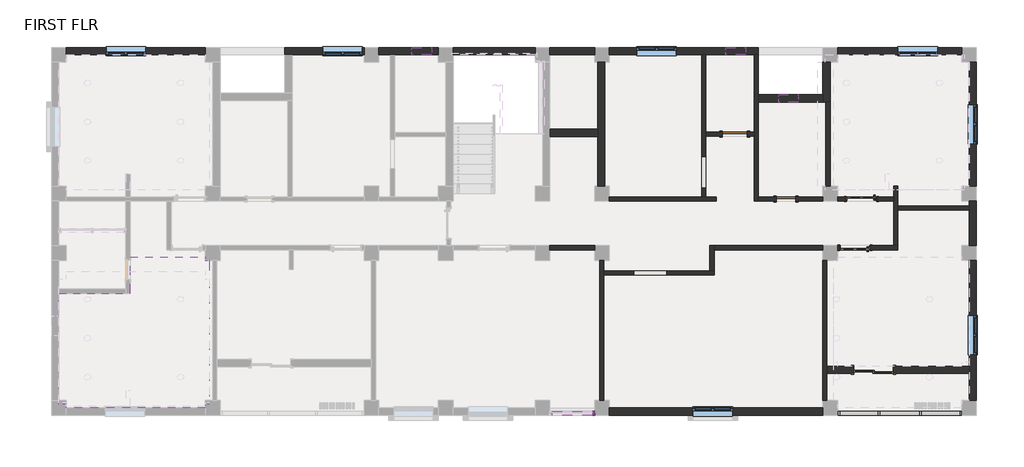
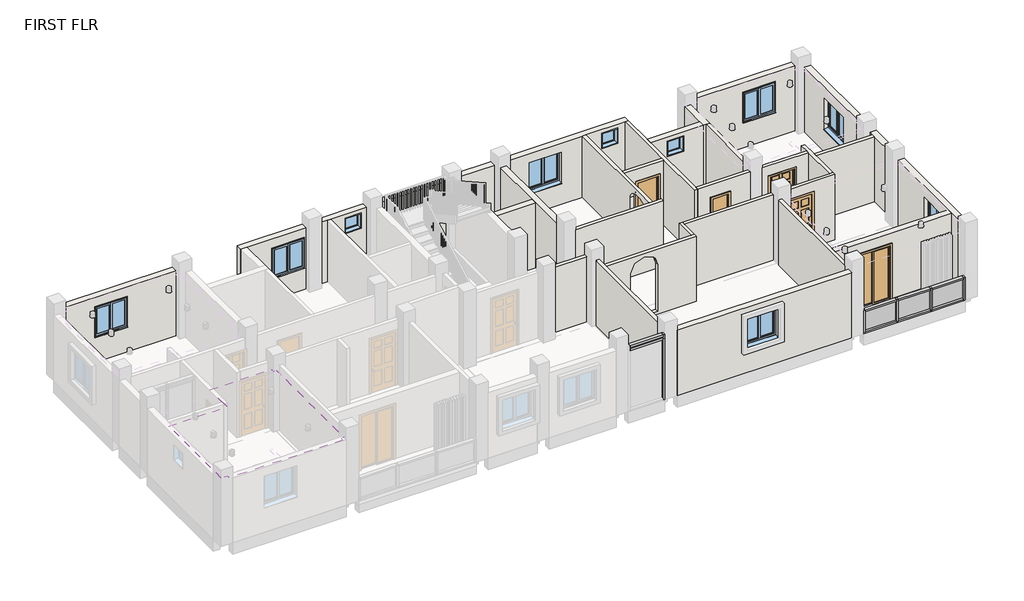
# One storey, part 2 of 5: 32 walls, 14 members, 10 windows, 5 doors, 3 plates, 1 covering.
"""IFC4 building model written with IfcOpenShell, lengths in millimetres."""

from ifc_helpers import new_model, si_unit, point, frame, origin, place, context, project, spatial, polyline, ellipse_curve, trimmed, outline, extrude, faceted_brep, transform, mapped, element, save
from ifc_brep_helpers import plane_surface, extruded_surface, advanced_brep
from components import door_double_sliding_4436dcad, door_c610b25b, door_03e3dfb5, single_flush_2_x_7_bath_room_door_025d1c86, door_1fe7f57d, member_5d96a33e, member_91edd790, member_ee409385, member_876f8f00, member_410c6227, member_73c23c35, member_71eb4692, member_a1da5be3, system_panel_glazed_2f542010, system_panel_glazed_876b4d55, window_80340324, w2_0001_4_x_4_window_9dec5fc7

model = new_model("IFC4")

# Units and contexts
model_context = context("Model", 3, world=origin())
ifc_project = project(units=[si_unit("LENGTHUNIT", "METRE", prefix="MILLI")], contexts=[model_context])

# Site, building, storey
site = spatial("IfcSite", under=ifc_project)
building = spatial("IfcBuilding", under=site)
storey = spatial("IfcBuildingStorey", under=building, Name="FIRST FLR", Elevation=3352.8)

# Covering
placement = place(None, origin())
element("IfcCovering", 1, ObjectType="GWB on Mtl. Stud", at=placement, inside=storey, context=model_context, shape_type="SweptSolid", body=[
    extrude(outline(polyline([(-15145.3456086, -10773.5679047), (-15145.3456086, -7363.1659448), (-12959.7401855, -7363.1659448), (-12959.7401855, -6244.0794704), (-10649.5456086, -6244.0794704), (-10649.5456086, -6358.3794704), (-10535.2456086, -6358.3794704), (-10535.2456086, -6963.5679047), (-10535.2456086, -10773.5679047), (-10649.5456086, -10773.5679047), (-10649.5456086, -10887.8679047), (-12959.7401855, -10887.8679047), (-14916.7456086, -10887.8679047), (-14916.7456086, -10773.5679047), (-15145.3456086, -10773.5679047)]), holes=[polyline([(-14840.5456086, -10583.0679047), (-10840.0456086, -10583.0679047), (-10840.0456086, -6548.8794704), (-12654.9401855, -6548.8794704), (-12654.9401855, -7667.9659448), (-14840.5456086, -7667.9659448), (-14840.5456086, -10583.0679047)])]), frame((0.0, 0.0, 5791.2), z_axis=(0.0, 0.0, 1.0), x_axis=(1.0, 0.0, 0.0)), (0.0, 0.0, 1.0), 107.95),
    extrude(outline(polyline([(-14688.1456086, -10430.6679047), (-14688.1456086, -7820.3659448), (-12502.5401855, -7820.3659448), (-12502.5401855, -6701.2794704), (-10992.4456086, -6701.2794704), (-10992.4456086, -10430.6679047), (-14688.1456086, -10430.6679047)]), holes=[polyline([(-14535.7456086, -7972.7659448), (-14535.7456086, -10278.2679047), (-11144.8456086, -10278.2679047), (-11144.8456086, -6853.6794704), (-12350.1401855, -6853.6794704), (-12350.1401855, -7972.7659448), (-14535.7456086, -7972.7659448)])]), frame((0.0, 0.0, 5791.2), z_axis=(0.0, 0.0, 1.0), x_axis=(1.0, 0.0, 0.0)), (0.0, 0.0, 1.0), 107.95),
])

# Doors
door_double_sliding_shape = door_double_sliding_4436dcad(model_context)
element("IfcDoor", 2, ObjectType="Door-Double-Sliding", at=placement, inside=storey, context=model_context, shape_type="MappedRepresentation", body=[
    mapped(door_double_sliding_shape, transform((9879.3128058, -9592.4679047, 3352.8), x_axis=(-1.0, 0.0, 0.0), y_axis=(0.0, -1.0, 0.0), z_axis=(0.0, 0.0, 1.0))),
])
door_shape = door_c610b25b(model_context)
element("IfcDoor", 3, ObjectType="Door-Interior-Single-6_Panel-Wood : 36\" x 84\"", at=placement, inside=storey, context=model_context, shape_type="MappedRepresentation", body=[
    mapped(door_shape, transform((9511.0128058, -4462.9044704, 3352.8), x_axis=(-1.0, 0.0, 0.0), y_axis=(0.0, -1.0, 0.0), z_axis=(0.0, 0.0, 1.0))),
])
door_2_shape = door_03e3dfb5(model_context)
element("IfcDoor", 4, ObjectType="Door-Interior-Single-6_Panel-Wood : 36\" x 84\"", at=placement, inside=storey, context=model_context, shape_type="MappedRepresentation", body=[
    mapped(door_2_shape, transform((9307.8128058, -5967.8544704, 3352.8), x_axis=(-1.0, 0.0, 0.0), y_axis=(0.0, -1.0, 0.0), z_axis=(0.0, 0.0, 1.0))),
])
single_flush_2_x_7_bath_room_door_shape = single_flush_2_x_7_bath_room_door_025d1c86(model_context)
element("IfcDoor", 5, ObjectType="Single-Flush : 2' X 7' BATH ROOM DOOR", at=placement, inside=storey, context=model_context, shape_type="MappedRepresentation", body=[
    mapped(single_flush_2_x_7_bath_room_door_shape, transform((7190.4916602, -4466.0794704, 3352.8), x_axis=(1.0, 0.0, 0.0), y_axis=(0.0, 1.0, 0.0), z_axis=(0.0, 0.0, 1.0))),
])
door_3_shape = door_1fe7f57d(model_context)
element("IfcDoor", 6, ObjectType="Single-Flush : 30\" x 80\"", at=placement, inside=storey, context=model_context, shape_type="MappedRepresentation", body=[
    mapped(door_3_shape, transform((5615.6916602, -2472.1794704, 3352.8), x_axis=(1.0, 0.0, 0.0), y_axis=(0.0, 1.0, 0.0), z_axis=(0.0, 0.0, 1.0))),
])

# Members
member_shape = member_5d96a33e(model_context)
element("IfcMember", 7, ObjectType="Rectangular Mullion : 2.5\" x 5\" rectangular", at=placement, inside=storey, context=model_context, shape_type="MappedRepresentation", body=[
    mapped(member_shape, transform((12520.9128058, -11052.9679047, 4267.2), x_axis=(0.0, 0.0, 1.0), y_axis=(0.0, -1.0, 0.0), z_axis=(1.0, 0.0, 0.0))),
])
element("IfcMember", 8, ObjectType="Rectangular Mullion : 2.5\" x 5\" rectangular", at=placement, inside=storey, context=model_context, shape_type="MappedRepresentation", body=[
    mapped(member_shape, transform((10012.6628059, -11052.9679047, 4267.2), x_axis=(0.0, 0.0, 1.0), y_axis=(0.0, -1.0, 0.0), z_axis=(1.0, 0.0, 0.0))),
])
element("IfcMember", 9, ObjectType="Rectangular Mullion : 2.5\" x 5\" rectangular", at=placement, inside=storey, context=model_context, shape_type="MappedRepresentation", body=[
    mapped(member_shape, transform((8837.9128058, -11052.9679047, 3352.8), x_axis=(0.0, 0.0, -1.0), y_axis=(0.0, -1.0, 0.0), z_axis=(-1.0, 0.0, 0.0))),
])
element("IfcMember", 10, ObjectType="Rectangular Mullion : 2.5\" x 5\" rectangular", at=placement, inside=storey, context=model_context, shape_type="MappedRepresentation", body=[
    mapped(member_shape, transform((11346.1628057, -11052.9679047, 3352.8), x_axis=(0.0, 0.0, -1.0), y_axis=(0.0, -1.0, 0.0), z_axis=(-1.0, 0.0, 0.0))),
])
member_2_shape = member_91edd790(model_context)
element("IfcMember", 11, ObjectType="Rectangular Mullion : 2.5\" x 5\" rectangular", at=placement, inside=storey, context=model_context, shape_type="MappedRepresentation", body=[
    mapped(member_2_shape, transform((11282.6628057, -11052.9679047, 4267.2), x_axis=(0.0, 0.0, 1.0), y_axis=(0.0, -1.0, 0.0), z_axis=(1.0, 0.0, 0.0))),
])
element("IfcMember", 12, ObjectType="Rectangular Mullion : 2.5\" x 5\" rectangular", at=placement, inside=storey, context=model_context, shape_type="MappedRepresentation", body=[
    mapped(member_2_shape, transform((10076.1628059, -11052.9679047, 3352.8), x_axis=(0.0, 0.0, -1.0), y_axis=(0.0, -1.0, 0.0), z_axis=(-1.0, 0.0, 0.0))),
])
member_3_shape = member_ee409385(model_context)
element("IfcMember", 13, ObjectType="Rectangular Mullion : 2.5\" x 5\" rectangular", at=placement, inside=storey, context=model_context, shape_type="MappedRepresentation", body=[
    mapped(member_3_shape, transform((1310.3916602, -11052.9679047, 3352.8), x_axis=(1.0, 0.0, 0.0), y_axis=(0.0, -1.0, 0.0), z_axis=(0.0, 0.0, -1.0))),
])
member_4_shape = member_876f8f00(model_context)
element("IfcMember", 14, ObjectType="Rectangular Mullion : 2.5\" x 5\" rectangular", at=placement, inside=storey, context=model_context, shape_type="MappedRepresentation", body=[
    mapped(member_4_shape, transform((1310.3916602, -11052.9679047, 5791.2), x_axis=(1.0, 0.0, 0.0), y_axis=(0.0, -1.0, 0.0), z_axis=(0.0, 0.0, -1.0))),
])
member_5_shape = member_410c6227(model_context)
element("IfcMember", 15, ObjectType="Rectangular Mullion : 2.5\" x 5\" rectangular", at=placement, inside=storey, context=model_context, shape_type="MappedRepresentation", body=[
    mapped(member_5_shape, transform((10044.4128059, -11052.9679047, 3352.8), x_axis=(1.0, 0.0, 0.0), y_axis=(0.0, -1.0, 0.0), z_axis=(0.0, 0.0, -1.0))),
])
element("IfcMember", 16, ObjectType="Rectangular Mullion : 2.5\" x 5\" rectangular", at=placement, inside=storey, context=model_context, shape_type="MappedRepresentation", body=[
    mapped(member_5_shape, transform((11314.4128057, -11052.9679047, 3352.8), x_axis=(1.0, 0.0, 0.0), y_axis=(0.0, -1.0, 0.0), z_axis=(0.0, 0.0, -1.0))),
])
member_6_shape = member_73c23c35(model_context)
element("IfcMember", 17, ObjectType="Rectangular Mullion : 2.5\" x 5\" rectangular", at=placement, inside=storey, context=model_context, shape_type="MappedRepresentation", body=[
    mapped(member_6_shape, transform((12584.4128058, -11052.9679047, 3352.8), x_axis=(1.0, 0.0, 0.0), y_axis=(0.0, -1.0, 0.0), z_axis=(0.0, 0.0, -1.0))),
])
element("IfcMember", 18, ObjectType="Rectangular Mullion : 2.5\" x 5\" rectangular", at=placement, inside=storey, context=model_context, shape_type="MappedRepresentation", body=[
    mapped(member_6_shape, transform((8774.4128058, -11052.9679047, 4267.2), x_axis=(-1.0, 0.0, 0.0), y_axis=(0.0, -1.0, 0.0), z_axis=(0.0, 0.0, 1.0))),
])
member_7_shape = member_71eb4692(model_context)
element("IfcMember", 19, ObjectType="Rectangular Mullion : 2.5\" x 5\" rectangular", at=placement, inside=storey, context=model_context, shape_type="MappedRepresentation", body=[
    mapped(member_7_shape, transform((1246.8916602, -11052.9679047, 5943.6), x_axis=(0.0, 0.0, 1.0), y_axis=(0.0, -1.0, 0.0), z_axis=(1.0, 0.0, 0.0))),
])
member_8_shape = member_a1da5be3(model_context)
element("IfcMember", 20, ObjectType="Rectangular Mullion : 2.5\" x 5\" rectangular", at=placement, inside=storey, context=model_context, shape_type="MappedRepresentation", body=[
    mapped(member_8_shape, transform((1246.8916602, -11052.9679047, 5791.2), x_axis=(0.0, 0.0, 1.0), y_axis=(0.0, -1.0, 0.0), z_axis=(1.0, 0.0, 0.0))),
])

# Plates
system_panel_glazed_shape = system_panel_glazed_2f542010(model_context)
element("IfcPlate", 21, ObjectType="System Panel : Glazed", at=placement, inside=storey, context=model_context, shape_type="MappedRepresentation", body=[
    mapped(system_panel_glazed_shape, transform((9425.2878058, -11052.9679047, 3416.3), x_axis=(1.0, 0.0, 0.0), y_axis=(0.0, 1.0, 0.0), z_axis=(0.0, 0.0, 1.0))),
])
element("IfcPlate", 22, ObjectType="System Panel : Glazed", at=placement, inside=storey, context=model_context, shape_type="MappedRepresentation", body=[
    mapped(system_panel_glazed_shape, transform((11933.5378057, -11052.9679047, 3416.3), x_axis=(1.0, 0.0, 0.0), y_axis=(0.0, 1.0, 0.0), z_axis=(0.0, 0.0, 1.0))),
])
system_panel_glazed_2_shape = system_panel_glazed_876b4d55(model_context)
element("IfcPlate", 23, ObjectType="System Panel : Glazed", at=placement, inside=storey, context=model_context, shape_type="MappedRepresentation", body=[
    mapped(system_panel_glazed_2_shape, transform((10679.4128058, -11052.9679047, 3416.3), x_axis=(1.0, 0.0, 0.0), y_axis=(0.0, 1.0, 0.0), z_axis=(0.0, 0.0, 1.0))),
])

# Walls
element("IfcWall", 24, ObjectType="EXTERIOR WALL 9\"", at=placement, inside=storey, context=model_context, shape_type="SweptSolid", body=[
    extrude(outline(polyline([(3352.8, 1767.5916602), (3352.8, 8317.2128058), (5943.6, 8317.2128058), (5943.6, 1767.5916602), (3352.8, 1767.5916602)]), holes=[polyline([(4352.8, 5552.1916602), (4352.8, 4332.9916602), (5572.0, 4332.9916602), (5572.0, 5552.1916602), (4352.8, 5552.1916602)])]), frame((0.0, -11116.4679047, 0.0), z_axis=(0.0, 1.0, 0.0), x_axis=(0.0, 0.0, 1.0)), (0.0, 0.0, 1.0), 228.6),
])
element("IfcWall", 25, ObjectType="EXTERIOR WALL 9\"", at=placement, inside=storey, context=model_context, shape_type="Brep", body=[
    faceted_brep([(13041.6128058, -10659.2679047, 3352.8), (13041.6128058, -6358.3794704, 3352.8), (13041.6128058, -6358.3794704, 5943.6), (13041.6128058, -10659.2679047, 5943.6), (13041.6128058, -9262.2679047, 4267.2), (13041.6128058, -9262.2679047, 5486.4), (13041.6128058, -8043.0679047, 5486.4), (13041.6128058, -8043.0679047, 4267.2), (12813.0128058, -10659.2679047, 3352.8), (12813.0128058, -10659.2679047, 5943.6), (12813.0128058, -9833.7679047, 5943.6), (12813.0128058, -9605.1679047, 5943.6), (12813.0128058, -6358.3794704, 5943.6), (12813.0128058, -6358.3794704, 3352.8), (12813.0128058, -9605.1679047, 3352.8), (12813.0128058, -9833.7679047, 3352.8), (12813.0128058, -9262.2679047, 4267.2), (12813.0128058, -8043.0679047, 4267.2), (12813.0128058, -8043.0679047, 5486.4), (12813.0128058, -9262.2679047, 5486.4)], [[[0, 1, 2, 3], [4, 5, 6, 7]], [[8, 9, 10, 11, 12, 13, 14, 15], [16, 17, 18, 19]], [[1, 0, 8, 15, 14, 13]], [[2, 1, 13, 12]], [[3, 2, 12, 11, 10, 9]], [[0, 3, 9, 8]], [[5, 4, 16, 19]], [[6, 5, 19, 18]], [[7, 6, 18, 17]], [[4, 7, 17, 16]]]),
])
element("IfcWall", 26, ObjectType="EXTERIOR WALL 9\"", at=placement, inside=storey, context=model_context, shape_type="Brep", body=[
    faceted_brep([(13041.6128058, -5901.1794704, 3352.8), (13041.6128058, -4529.5794704, 3352.8), (13041.6128058, -4529.5794704, 5943.6), (13041.6128058, -5901.1794704, 5943.6), (12813.0128058, -5901.1794704, 3352.8), (12813.0128058, -5901.1794704, 5943.6), (12813.0128058, -4808.9794704, 5943.6), (12813.0128058, -4681.9794704, 5943.6), (12813.0128058, -4529.5794704, 5943.6), (12813.0128058, -4529.5794704, 3352.8), (12813.0128058, -4681.9794704, 3352.8), (12813.0128058, -4808.9794704, 3352.8)], [[[0, 1, 2, 3]], [[4, 5, 6, 7, 8, 9, 10, 11]], [[1, 0, 4, 11, 10, 9]], [[2, 1, 9, 8]], [[3, 2, 8, 7, 6, 5]], [[0, 3, 5, 4]]]),
])
element("IfcWall", 27, ObjectType="EXTERIOR WALL 9\"", at=placement, inside=storey, context=model_context, shape_type="SweptSolid", body=[
    extrude(outline(polyline([(-4072.3794704, 3352.8), (-4072.3794704, 5943.6), (-262.3794704, 5943.6), (-262.3794704, 3352.8), (-4072.3794704, 3352.8)]), holes=[polyline([(-2776.9794704, 4267.2), (-1557.7794704, 4267.2), (-1557.7794704, 5486.4), (-2776.9794704, 5486.4), (-2776.9794704, 4267.2)])]), frame((12813.0128058, 0.0, 0.0), z_axis=(1.0, 0.0, 0.0), x_axis=(0.0, 1.0, 0.0)), (0.0, 0.0, 1.0), 228.6),
])
element("IfcWall", 28, ObjectType="EXTERIOR WALL 9\"", at=placement, inside=storey, context=model_context, shape_type="SweptSolid", body=[
    extrude(outline(polyline([(3352.8, 12584.4128058), (5943.6, 12584.4128058), (5943.6, 8774.4128058), (3352.8, 8774.4128058), (3352.8, 12584.4128058)]), holes=[polyline([(4352.8, 10628.6128058), (5572.0, 10628.6128058), (5572.0, 11847.8128058), (4352.8, 11847.8128058), (4352.8, 10628.6128058)])]), frame((0.0, -33.7794704, 0.0), z_axis=(0.0, 1.0, 0.0), x_axis=(0.0, 0.0, 1.0)), (0.0, 0.0, 1.0), 228.6),
])
element("IfcWall", 29, ObjectType="EXTERIOR WALL 9\"", at=placement, inside=storey, context=model_context, shape_type="SweptSolid", body=[
    extrude(outline(polyline([(3352.8, -14916.7456086), (3352.8, -10649.5456086), (5943.6, -10649.5456086), (5943.6, -14916.7456086), (3352.8, -14916.7456086)]), holes=[polyline([(4352.8, -13697.5456086), (5572.0, -13697.5456086), (5572.0, -12478.3456086), (4352.8, -12478.3456086), (4352.8, -13697.5456086)])]), frame((0.0, -33.7794704, 0.0), z_axis=(0.0, 1.0, 0.0), x_axis=(0.0, 0.0, 1.0)), (0.0, 0.0, 1.0), 228.6),
])
element("IfcWall", 30, ObjectType="EXTERIOR WALL 9\"", at=placement, inside=storey, context=model_context, shape_type="SweptSolid", body=[
    extrude(outline(polyline([(3352.8, 8444.2128058), (3352.8, 9269.7128058), (5486.4, 9269.7128058), (5486.4, 10488.9128058), (3352.8, 10488.9128058), (3352.8, 12813.0128058), (5943.6, 12813.0128058), (5943.6, 8444.2128058), (3352.8, 8444.2128058)])), frame((0.0, -9833.7679047, 0.0), z_axis=(0.0, 1.0, 0.0), x_axis=(0.0, 0.0, 1.0)), (0.0, 0.0, 1.0), 228.6),
])
element("IfcWall", 31, ObjectType="EXTERIOR WALL 9\"", at=placement, inside=storey, context=model_context, shape_type="Brep", body=[
    faceted_brep([(-5772.7456086, 194.8205296, 3352.8), (-8211.1456086, 194.8205296, 3352.8), (-8211.1456086, 194.8205296, 5943.6), (-5772.7456086, 194.8205296, 5943.6), (-7042.7456086, 194.8205296, 4352.8), (-5823.5456086, 194.8205296, 4352.8), (-5823.5456086, 194.8205296, 5572.0), (-7042.7456086, 194.8205296, 5572.0), (-5772.7456086, -33.7794704, 3352.8), (-5772.7456086, -33.7794704, 5943.6), (-7982.5456086, -33.7794704, 5943.6), (-8211.1456086, -33.7794704, 5943.6), (-8211.1456086, -33.7794704, 3352.8), (-7982.5456086, -33.7794704, 3352.8), (-7042.7456086, -33.7794704, 4352.8), (-7042.7456086, -33.7794704, 5572.0), (-5823.5456086, -33.7794704, 5572.0), (-5823.5456086, -33.7794704, 4352.8)], [[[0, 1, 2, 3], [4, 5, 6, 7]], [[8, 9, 10, 11, 12, 13], [14, 15, 16, 17]], [[1, 0, 8, 13, 12]], [[3, 2, 11, 10, 9]], [[0, 3, 9, 8]], [[2, 1, 12, 11]], [[15, 14, 4, 7]], [[16, 15, 7, 6]], [[17, 16, 6, 5]], [[14, 17, 5, 4]]]),
])
element("IfcWall", 32, ObjectType="EXTERIOR WALL 9\"", at=placement, inside=storey, context=model_context, shape_type="Brep", body=[
    faceted_brep([(-5315.5456086, -33.7794704, 3352.8), (-4959.9456086, -33.7794704, 3352.8), (-4832.9456086, -33.7794704, 3352.8), (-3486.7456086, -33.7794704, 3352.8), (-3486.7456086, -33.7794704, 5943.6), (-4832.9456086, -33.7794704, 5943.6), (-4959.9456086, -33.7794704, 5943.6), (-5315.5456086, -33.7794704, 5943.6), (-3689.9456086, -33.7794704, 5791.2), (-3689.9456086, -33.7794704, 5181.6), (-4299.5456086, -33.7794704, 5181.6), (-4299.5456086, -33.7794704, 5791.2), (-3486.7456086, 194.8205296, 3352.8), (-5315.5456086, 194.8205296, 3352.8), (-5315.5456086, 194.8205296, 5943.6), (-3486.7456086, 194.8205296, 5943.6), (-3689.9456086, 194.8205296, 5181.6), (-3689.9456086, 194.8205296, 5791.2), (-4299.5456086, 194.8205296, 5791.2), (-4299.5456086, 194.8205296, 5181.6)], [[[0, 1, 2, 3, 4, 5, 6, 7], [8, 9, 10, 11]], [[12, 13, 14, 15], [16, 17, 18, 19]], [[3, 2, 1, 0, 13, 12]], [[4, 3, 12, 15]], [[7, 6, 5, 4, 15, 14]], [[0, 7, 14, 13]], [[8, 17, 16, 9]], [[9, 16, 19, 10]], [[10, 19, 18, 11]], [[17, 8, 11, 18]]]),
])
element("IfcWall", 33, ObjectType="EXTERIOR WALL 9\"", at=placement, inside=storey, context=model_context, shape_type="SweptSolid", body=[
    extrude(outline(polyline([(-518.4083398, -33.7794704), (-3029.5456086, -33.7794704), (-3029.5456086, 194.8205296), (-518.4083398, 194.8205296), (-518.4083398, -33.7794704)])), frame((0.0, 0.0, 3352.8), z_axis=(0.0, 0.0, 1.0), x_axis=(1.0, 0.0, 0.0)), (0.0, 0.0, 1.0), 2590.8),
])
element("IfcWall", 34, ObjectType="EXTERIOR WALL 9\"", at=placement, inside=storey, context=model_context, shape_type="SweptSolid", body=[
    extrude(outline(polyline([(1310.3916602, -33.7794704), (-61.2083398, -33.7794704), (-61.2083398, 194.8205296), (1310.3916602, 194.8205296), (1310.3916602, -33.7794704)])), frame((0.0, 0.0, 3352.8), z_axis=(0.0, 0.0, 1.0), x_axis=(1.0, 0.0, 0.0)), (0.0, 0.0, 1.0), 2590.8),
])
element("IfcWall", 35, ObjectType="EXTERIOR WALL 9\"", at=placement, inside=storey, context=model_context, shape_type="Brep", body=[
    faceted_brep([(1767.5916602, -33.7794704, 3352.8), (4599.6916602, -33.7794704, 3352.8), (4726.6916602, -33.7794704, 3352.8), (6212.5916602, -33.7794704, 3352.8), (6339.5916602, -33.7794704, 3352.8), (6339.5916602, -33.7794704, 5943.6), (6212.5916602, -33.7794704, 5943.6), (4726.6916602, -33.7794704, 5943.6), (4599.6916602, -33.7794704, 5943.6), (1767.5916602, -33.7794704, 5943.6), (3824.9916602, -33.7794704, 5572.0), (3824.9916602, -33.7794704, 4352.8), (2605.7916602, -33.7794704, 4352.8), (2605.7916602, -33.7794704, 5572.0), (5945.8916602, -33.7794704, 5791.2), (5945.8916602, -33.7794704, 5181.6), (5336.2916602, -33.7794704, 5181.6), (5336.2916602, -33.7794704, 5791.2), (6339.5916602, 194.8205296, 3352.8), (1767.5916602, 194.8205296, 3352.8), (1767.5916602, 194.8205296, 5943.6), (6339.5916602, 194.8205296, 5943.6), (3824.9916602, 194.8205296, 4352.8), (3824.9916602, 194.8205296, 5572.0), (2605.7916602, 194.8205296, 5572.0), (2605.7916602, 194.8205296, 4352.8), (5945.8916602, 194.8205296, 5181.6), (5945.8916602, 194.8205296, 5791.2), (5336.2916602, 194.8205296, 5791.2), (5336.2916602, 194.8205296, 5181.6)], [[[0, 1, 2, 3, 4, 5, 6, 7, 8, 9], [10, 11, 12, 13], [14, 15, 16, 17]], [[18, 19, 20, 21], [22, 23, 24, 25], [26, 27, 28, 29]], [[4, 3, 2, 1, 0, 19, 18]], [[9, 8, 7, 6, 5, 21, 20]], [[0, 9, 20, 19]], [[5, 4, 18, 21]], [[23, 22, 11, 10]], [[24, 23, 10, 13]], [[25, 24, 13, 12]], [[22, 25, 12, 11]], [[14, 27, 26, 15]], [[15, 26, 29, 16]], [[16, 29, 28, 17]], [[27, 14, 17, 28]]]),
])
element("IfcWall", 36, ObjectType="EXTERIOR WALL 9\"", at=placement, inside=storey, context=model_context, shape_type="Brep", body=[
    faceted_brep([(8317.2128058, -262.3794704, 3352.8), (8317.2128058, -1252.9794704, 3352.8), (8317.2128058, -1481.5794704, 3352.8), (8317.2128058, -1481.5794704, 5943.6), (8317.2128058, -1252.9794704, 5943.6), (8317.2128058, -262.3794704, 5943.6), (8545.8128058, -262.3794704, 3352.8), (8545.8128058, -262.3794704, 5943.6), (8545.8128058, -1481.5794704, 5943.6), (8545.8128058, -1481.5794704, 3352.8), (8418.8128058, -1481.5794704, 3352.8), (8418.8128058, -1481.5794704, 5943.6)], [[[0, 1, 2, 3, 4, 5]], [[6, 7, 8, 9]], [[2, 1, 0, 6, 9, 10]], [[5, 4, 3, 11, 8, 7]], [[0, 5, 7, 6]], [[3, 2, 10, 9, 8, 11]]]),
])
element("IfcWall", 37, ObjectType="EXTERIOR WALL 9\"", at=placement, inside=storey, context=model_context, shape_type="SweptSolid", body=[
    extrude(outline(polyline([(3352.8, 6339.5916602), (3352.8, 8317.2128058), (5943.6, 8317.2128058), (5943.6, 6339.5916602), (3352.8, 6339.5916602)]), holes=[polyline([(5791.2, 7571.4916602), (5181.6, 7571.4916602), (5181.6, 6961.8916602), (5791.2, 6961.8916602), (5791.2, 7571.4916602)])]), frame((0.0, -1481.5794704, 0.0), z_axis=(0.0, 1.0, 0.0), x_axis=(0.0, 0.0, 1.0)), (0.0, 0.0, 1.0), 228.6),
])
element("IfcWall", 38, ObjectType="EXTERIOR WALL 9\"", at=placement, inside=storey, context=model_context, shape_type="Brep", body=[
    faceted_brep([(1399.2916602, -262.3794704, 3352.8), (1399.2916602, -2319.7794704, 3352.8), (1399.2916602, -2548.3794704, 3352.8), (1399.2916602, -4072.3794704, 3352.8), (1399.2916602, -4072.3794704, 5943.6), (1399.2916602, -2548.3794704, 5943.6), (1399.2916602, -2319.7794704, 5943.6), (1399.2916602, -262.3794704, 5943.6), (1627.8916602, -262.3794704, 3352.8), (1627.8916602, -262.3794704, 5943.6), (1627.8916602, -4072.3794704, 5943.6), (1627.8916602, -4072.3794704, 3352.8)], [[[0, 1, 2, 3, 4, 5, 6, 7]], [[8, 9, 10, 11]], [[3, 2, 1, 0, 8, 11]], [[4, 3, 11, 10]], [[7, 6, 5, 4, 10, 9]], [[0, 7, 9, 8]]]),
])
element("IfcWall", 39, ObjectType="EXTERIOR WALL 9\"", at=placement, inside=storey, context=model_context, shape_type="SweptSolid", body=[
    extrude(outline(polyline([(1399.2916602, -2548.3794704), (-61.2083398, -2548.3794704), (-61.2083398, -2319.7794704), (1399.2916602, -2319.7794704), (1399.2916602, -2548.3794704)])), frame((0.0, 0.0, 3352.8), z_axis=(0.0, 0.0, 1.0), x_axis=(1.0, 0.0, 0.0)), (0.0, 0.0, 1.0), 2590.8),
])
element("IfcWall", 40, ObjectType="INTERIOR WALL 5\"", at=placement, inside=storey, context=model_context, shape_type="Brep", body=[
    faceted_brep([(1589.7916602, -10659.2679047, 3352.8), (1589.7916602, -6802.8794704, 3352.8), (1589.7916602, -6675.8794704, 3352.8), (1589.7916602, -6358.3794704, 3352.8), (1589.7916602, -6358.3794704, 5943.6), (1589.7916602, -6675.8794704, 5943.6), (1589.7916602, -6802.8794704, 5943.6), (1589.7916602, -10659.2679047, 5943.6), (1462.7916602, -10659.2679047, 3352.8), (1462.7916602, -10659.2679047, 5943.6), (1462.7916602, -6358.3794704, 5943.6), (1462.7916602, -6358.3794704, 3352.8)], [[[0, 1, 2, 3, 4, 5, 6, 7]], [[8, 9, 10, 11]], [[3, 2, 1, 0, 8, 11]], [[4, 3, 11, 10]], [[7, 6, 5, 4, 10, 9]], [[0, 7, 9, 8]]]),
])
element("IfcWall", 41, ObjectType="INTERIOR WALL 5\"", at=placement, inside=storey, context=model_context, shape_type="Brep", body=[
    faceted_brep([(8444.2128058, -10659.2679047, 3352.8), (8444.2128058, -9833.7679047, 3352.8), (8444.2128058, -9605.1679047, 3352.8), (8444.2128058, -6358.3794704, 3352.8), (8444.2128058, -6358.3794704, 5943.6), (8444.2128058, -9605.1679047, 5943.6), (8444.2128058, -9833.7679047, 5943.6), (8444.2128058, -10659.2679047, 5943.6), (8317.2128058, -10659.2679047, 3352.8), (8317.2128058, -10659.2679047, 5943.6), (8317.2128058, -6358.3794704, 5943.6), (8317.2128058, -6358.3794704, 3352.8)], [[[0, 1, 2, 3, 4, 5, 6, 7]], [[8, 9, 10, 11]], [[3, 2, 1, 0, 8, 11]], [[4, 3, 11, 10]], [[7, 6, 5, 4, 10, 9]], [[0, 7, 9, 8]]]),
])
element("IfcWall", 42, ObjectType="INTERIOR WALL 5\"", at=placement, inside=storey, context=model_context, shape_type="SweptSolid", body=[
    extrude(outline(polyline([(10628.6128058, -4681.9794704), (12813.0128058, -4681.9794704), (12813.0128058, -4808.9794704), (10628.6128058, -4808.9794704), (10628.6128058, -4681.9794704)])), frame((0.0, 0.0, 3352.8), z_axis=(0.0, 0.0, 1.0), x_axis=(1.0, 0.0, 0.0)), (0.0, 0.0, 1.0), 2590.8),
])
element("IfcWall", 43, ObjectType="INTERIOR WALL 5\"", at=placement, inside=storey, context=model_context, shape_type="Brep", body=[
    faceted_brep([(10628.6128058, -6028.1794704, 5943.6), (8774.4128058, -6028.1794704, 5943.6), (8774.4128058, -6028.1794704, 3352.8), (8825.2128058, -6028.1794704, 3352.8), (8825.2128058, -6028.1794704, 5511.8), (9790.4128058, -6028.1794704, 5511.8), (9790.4128058, -6028.1794704, 3352.8), (10628.6128058, -6028.1794704, 3352.8), (8774.4128058, -5901.1794704, 5943.6), (10501.6128058, -5901.1794704, 5943.6), (10628.6128058, -5901.1794704, 5943.6), (10628.6128058, -5901.1794704, 3352.8), (10501.6128058, -5901.1794704, 3352.8), (9790.4128058, -5901.1794704, 3352.8), (9790.4128058, -5901.1794704, 5511.8), (8825.2128058, -5901.1794704, 5511.8), (8825.2128058, -5901.1794704, 3352.8), (8774.4128058, -5901.1794704, 3352.8)], [[[0, 1, 2, 3, 4, 5, 6, 7]], [[8, 9, 10, 11, 12, 13, 14, 15, 16, 17]], [[2, 17, 16, 3]], [[11, 7, 6, 13, 12]], [[1, 0, 10, 9, 8]], [[2, 1, 8, 17]], [[0, 7, 11, 10]], [[15, 4, 3, 16]], [[4, 15, 14, 5]], [[5, 14, 13, 6]]]),
])
element("IfcWall", 44, ObjectType="INTERIOR WALL 5\"", at=placement, inside=storey, context=model_context, shape_type="Brep", body=[
    faceted_brep([(10628.6128058, -5901.1794704, 3352.8), (10628.6128058, -4808.9794704, 3352.8), (10628.6128058, -4681.9794704, 3352.8), (10628.6128058, -4072.3794704, 3352.8), (10628.6128058, -4072.3794704, 5943.6), (10628.6128058, -4681.9794704, 5943.6), (10628.6128058, -4808.9794704, 5943.6), (10628.6128058, -5901.1794704, 5943.6), (10501.6128058, -5901.1794704, 3352.8), (10501.6128058, -5901.1794704, 5943.6), (10501.6128058, -4529.5794704, 5943.6), (10501.6128058, -4402.5794704, 5943.6), (10501.6128058, -4072.3794704, 5943.6), (10501.6128058, -4072.3794704, 3352.8), (10501.6128058, -4402.5794704, 3352.8), (10501.6128058, -4529.5794704, 3352.8)], [[[0, 1, 2, 3, 4, 5, 6, 7]], [[8, 9, 10, 11, 12, 13, 14, 15]], [[3, 2, 1, 0, 8, 15, 14, 13]], [[4, 3, 13, 12]], [[7, 6, 5, 4, 12, 11, 10, 9]], [[0, 7, 9, 8]]]),
])
element("IfcWall", 45, ObjectType="INTERIOR WALL 5\"", at=placement, inside=storey, context=model_context, shape_type="Brep", body=[
    faceted_brep([(6212.5916602, -33.7794704, 3352.8), (6212.5916602, -2408.6794704, 3352.8), (6212.5916602, -2535.6794704, 3352.8), (6212.5916602, -4529.5794704, 3352.8), (6212.5916602, -4529.5794704, 5943.6), (6212.5916602, -2535.6794704, 5943.6), (6212.5916602, -2408.6794704, 5943.6), (6212.5916602, -33.7794704, 5943.6), (6339.5916602, -33.7794704, 3352.8), (6339.5916602, -33.7794704, 5943.6), (6339.5916602, -1252.9794704, 5943.6), (6339.5916602, -1481.5794704, 5943.6), (6339.5916602, -4402.5794704, 5943.6), (6339.5916602, -4529.5794704, 5943.6), (6339.5916602, -4529.5794704, 3352.8), (6339.5916602, -4402.5794704, 3352.8), (6339.5916602, -1481.5794704, 3352.8), (6339.5916602, -1252.9794704, 3352.8)], [[[0, 1, 2, 3, 4, 5, 6, 7]], [[8, 9, 10, 11, 12, 13, 14, 15, 16, 17]], [[3, 2, 1, 0, 8, 17, 16, 15, 14]], [[7, 6, 5, 4, 13, 12, 11, 10, 9]], [[0, 7, 9, 8]], [[4, 3, 14, 13]]]),
])
element("IfcWall", 46, ObjectType="INTERIOR WALL 5\"", at=placement, inside=storey, context=model_context, shape_type="SweptSolid", body=[
    extrude(outline(polyline([(8418.8128058, -4072.3794704), (8418.8128058, -1481.5794704), (8545.8128058, -1481.5794704), (8545.8128058, -4072.3794704), (8418.8128058, -4072.3794704)])), frame((0.0, 0.0, 3352.8), z_axis=(0.0, 0.0, 1.0), x_axis=(1.0, 0.0, 0.0)), (0.0, 0.0, 1.0), 2590.8),
])
element("IfcWall", 47, ObjectType="INTERIOR WALL 5\"", at=placement, inside=storey, context=model_context, shape_type="Brep", body=[
    faceted_brep([(1767.5916602, -4529.5794704, 3352.8), (5044.1916602, -4529.5794704, 3352.8), (5044.1916602, -4529.5794704, 5943.6), (1767.5916602, -4529.5794704, 5943.6), (1767.5916602, -4402.5794704, 3352.8), (1767.5916602, -4402.5794704, 5943.6), (4599.6916602, -4402.5794704, 5943.6), (4726.6916602, -4402.5794704, 5943.6), (5044.1916602, -4402.5794704, 5943.6), (5044.1916602, -4402.5794704, 3352.8), (4726.6916602, -4402.5794704, 3352.8), (4599.6916602, -4402.5794704, 3352.8)], [[[0, 1, 2, 3]], [[4, 5, 6, 7, 8, 9, 10, 11]], [[1, 0, 4, 11, 10, 9]], [[2, 1, 9, 8]], [[3, 2, 8, 7, 6, 5]], [[0, 3, 5, 4]]]),
])
element("IfcWall", 48, ObjectType="INTERIOR WALL 5\"", at=placement, inside=storey, context=model_context, shape_type="AdvancedBrep", body=[
    advanced_brep(
    [(4599.6916602, -33.7794704, 3352.8), (4599.6916602, -4402.5794704, 3352.8), (4599.6916602, -4402.5794704, 5943.6), (4599.6916602, -33.7794704, 5943.6), (4599.6916602, -3162.9760679, 5411.4701015), (4599.6916602, -4128.1760679, 5411.4701015), (4599.6916602, -4128.1760679, 3531.8701015), (4599.6916602, -3162.9760679, 3531.8701015), (4726.6916602, -33.7794704, 3352.8), (4726.6916602, -33.7794704, 5943.6), (4726.6916602, -2408.6794704, 5943.6), (4726.6916602, -2535.6794704, 5943.6), (4726.6916602, -4402.5794704, 5943.6), (4726.6916602, -4402.5794704, 3352.8), (4726.6916602, -2535.6794704, 3352.8), (4726.6916602, -2408.6794704, 3352.8), (4726.6916602, -3162.9760679, 5411.4701015), (4726.6916602, -3162.9760679, 3531.8701015), (4726.6916602, -4128.1760679, 3531.8701015), (4726.6916602, -4128.1760679, 5411.4701015)],
    [
        (0, 1),
        (1, 2),
        (2, 3),
        (3, 0),
        (4, 5, ellipse_curve(frame((4599.6916602, -3645.5760679, 5411.4701015), z_axis=(1.0, 0.0, 0.0), x_axis=(0.0, -1.0, 0.0)), 482.6, 330.2)),
        (5, 6),
        (6, 7),
        (7, 4),
        (8, 9),
        (9, 10),
        (10, 11),
        (11, 12),
        (12, 13),
        (13, 14),
        (14, 15),
        (15, 8),
        (16, 17),
        (17, 18),
        (18, 19),
        (19, 16, ellipse_curve(frame((4726.6916602, -3645.5760679, 5411.4701015), z_axis=(-1.0, 0.0, 0.0), x_axis=(0.0, -1.0, 0.0)), 482.6, 330.2)),
        (3, 9),
        (8, 0),
        (1, 13),
        (12, 2),
        (4, 16),
        (19, 5),
        (18, 6),
        (17, 7),
    ],
    [
        plane_surface(frame((4599.6916602, 80.5205296, 3352.8), z_axis=(-1.0, 0.0, 0.0), x_axis=(0.0, -1.0, 0.0))),
        plane_surface(frame((4726.6916602, 80.5205296, 3352.8), z_axis=(1.0, 0.0, 0.0), x_axis=(0.0, 1.0, 0.0))),
        plane_surface(frame((1784.6412895, -33.7794704, 3352.8), z_axis=(0.0, 1.0, 0.0), x_axis=(1.0, 0.0, 0.0))),
        plane_surface(frame((1767.5916602, -4402.5794704, 3352.8), z_axis=(0.0, -1.0, 0.0), x_axis=(-1.0, 0.0, 0.0))),
        plane_surface(frame((4599.6916602, 80.5205296, 3352.8), z_axis=(0.0, 0.0, -1.0), x_axis=(1.0, 0.0, 0.0))),
        plane_surface(frame((4599.6916602, -4466.0794704, 5943.6), z_axis=(0.0, 0.0, 1.0), x_axis=(1.0, 0.0, 0.0))),
        extruded_surface(trimmed(ellipse_curve(frame((4790.1916602, -3645.5760679, 5411.4701015), z_axis=(1.0, 0.0, 0.0), x_axis=(0.0, -1.0, 0.0)), 482.6, 330.2), [point((4790.1916602, -3162.9760679, 5411.4701015))], [point((4790.1916602, -4128.1760679, 5411.4701015))], True, "CARTESIAN"), (-127.0, 0.0, 0.0), 127.0),
        plane_surface(frame((4599.6916602, -4128.1760679, 5411.4701015), z_axis=(0.0, 1.0, 0.0), x_axis=(1.0, 0.0, 0.0))),
        plane_surface(frame((4599.6916602, -4128.1760679, 3531.8701015), z_axis=(0.0, 0.0, 1.0), x_axis=(1.0, 0.0, 0.0))),
        plane_surface(frame((4599.6916602, -3162.9760679, 3531.8701015), z_axis=(0.0, -1.0, 0.0), x_axis=(1.0, 0.0, 0.0))),
    ],
    [
        (0, [[1, 2, 3, 4], [5, 6, 7, 8]]),
        (1, [[9, 10, 11, 12, 13, 14, 15, 16], [17, 18, 19, 20]]),
        (2, [[-4, 21, -9, 22]]),
        (3, [[-2, 23, -13, 24]]),
        (4, [[-1, -22, -16, -15, -14, -23]]),
        (5, [[-3, -24, -12, -11, -10, -21]]),
        (6, [[-5, 25, -20, 26]]),
        (7, [[-6, -26, -19, 27]]),
        (8, [[-7, -27, -18, 28]]),
        (9, [[-8, -28, -17, -25]]),
    ],
),
])
element("IfcWall", 49, ObjectType="INTERIOR WALL 5\"", at=placement, inside=storey, context=model_context, shape_type="SweptSolid", body=[
    extrude(outline(polyline([(5384.8, 5996.6916602), (3352.8, 5996.6916602), (3352.8, 6212.5916602), (5943.6, 6212.5916602), (5943.6, 4726.6916602), (3352.8, 4726.6916602), (3352.8, 5234.6916602), (5384.8, 5234.6916602), (5384.8, 5996.6916602)])), frame((0.0, -2535.6794704, 0.0), z_axis=(0.0, 1.0, 0.0), x_axis=(0.0, 0.0, 1.0)), (0.0, 0.0, 1.0), 127.0),
])
element("IfcWall", 50, ObjectType="INTERIOR WALL 5\"", at=placement, inside=storey, context=model_context, shape_type="SweptSolid", body=[
    extrude(outline(polyline([(5384.8, 7495.2916602), (3352.8, 7495.2916602), (3352.8, 8317.2128058), (5943.6, 8317.2128058), (5943.6, 6339.5916602), (3352.8, 6339.5916602), (3352.8, 6885.6916602), (5384.8, 6885.6916602), (5384.8, 7495.2916602)])), frame((0.0, -4529.5794704, 0.0), z_axis=(0.0, 1.0, 0.0), x_axis=(0.0, 0.0, 1.0)), (0.0, 0.0, 1.0), 127.0),
])
element("IfcWall", 51, ObjectType="INTERIOR WALL 5\"", at=placement, inside=storey, context=model_context, shape_type="SweptSolid", body=[
    extrude(outline(polyline([(5943.6, 10501.6128058), (5943.6, 8774.4128058), (3352.8, 8774.4128058), (3352.8, 9028.4128058), (5511.8, 9028.4128058), (5511.8, 9993.6128058), (3352.8, 9993.6128058), (3352.8, 10501.6128058), (5943.6, 10501.6128058)])), frame((0.0, -4529.5794704, 0.0), z_axis=(0.0, 1.0, 0.0), x_axis=(0.0, 0.0, 1.0)), (0.0, 0.0, 1.0), 127.0),
])
element("IfcWall", 52, ObjectType="INTERIOR WALL 5\"", at=placement, inside=storey, context=model_context, shape_type="SweptSolid", body=[
    extrude(outline(polyline([(-61.2083398, -5901.1794704), (1310.3916602, -5901.1794704), (1310.3916602, -6028.1794704), (-61.2083398, -6028.1794704), (-61.2083398, -5901.1794704)])), frame((0.0, 0.0, 3352.8), z_axis=(0.0, 0.0, 1.0), x_axis=(1.0, 0.0, 0.0)), (0.0, 0.0, 1.0), 2590.8),
])
element("IfcWall", 53, ObjectType="INTERIOR WALL 5\"", at=placement, inside=storey, context=model_context, shape_type="AdvancedBrep", body=[
    advanced_brep(
    [(1589.7916602, -6802.8794704, 3352.8), (4980.6916602, -6802.8794704, 3352.8), (4980.6916602, -6802.8794704, 5943.6), (1589.7916602, -6802.8794704, 5943.6), (2514.6258025, -6802.8794704, 5315.5597277), (3530.6258025, -6802.8794704, 5315.5597277), (3530.6258025, -6802.8794704, 3461.3597277), (2514.6258025, -6802.8794704, 3461.3597277), (1589.7916602, -6675.8794704, 3352.8), (1589.7916602, -6675.8794704, 5943.6), (4853.6916602, -6675.8794704, 5943.6), (4980.6916602, -6675.8794704, 5943.6), (4980.6916602, -6675.8794704, 3352.8), (4853.6916602, -6675.8794704, 3352.8), (2514.6258025, -6675.8794704, 5315.5597277), (2514.6258025, -6675.8794704, 3461.3597277), (3530.6258025, -6675.8794704, 3461.3597277), (3530.6258025, -6675.8794704, 5315.5597277)],
    [
        (0, 1),
        (1, 2),
        (2, 3),
        (3, 0),
        (4, 5, ellipse_curve(frame((3022.6258025, -6802.8794704, 5315.5597277), z_axis=(0.0, 1.0, 0.0), x_axis=(-1.0, 0.0, 0.0)), 508.0, 482.6)),
        (5, 6),
        (6, 7),
        (7, 4),
        (8, 9),
        (9, 10),
        (10, 11),
        (11, 12),
        (12, 13),
        (13, 8),
        (14, 15),
        (15, 16),
        (16, 17),
        (17, 14, ellipse_curve(frame((3022.6258025, -6675.8794704, 5315.5597277), z_axis=(0.0, -1.0, 0.0), x_axis=(-1.0, 0.0, 0.0)), 508.0, 482.6)),
        (3, 9),
        (8, 0),
        (1, 12),
        (11, 2),
        (4, 14),
        (17, 5),
        (16, 6),
        (15, 7),
    ],
    [
        plane_surface(frame((1526.2916602, -6802.8794704, 3352.8), z_axis=(0.0, -1.0, 0.0), x_axis=(1.0, 0.0, 0.0))),
        plane_surface(frame((1526.2916602, -6675.8794704, 3352.8), z_axis=(0.0, 1.0, 0.0), x_axis=(-1.0, 0.0, 0.0))),
        plane_surface(frame((1589.7916602, -10648.7570633, 3352.8), z_axis=(-1.0, 0.0, 0.0), x_axis=(0.0, 1.0, 0.0))),
        plane_surface(frame((4980.6916602, -6675.8794704, 3352.8), z_axis=(1.0, 0.0, 0.0), x_axis=(0.0, 1.0, 0.0))),
        plane_surface(frame((1526.2916602, -6802.8794704, 3352.8), z_axis=(0.0, 0.0, -1.0), x_axis=(0.0, 1.0, 0.0))),
        plane_surface(frame((4917.1916602, -6802.8794704, 5943.6), z_axis=(0.0, 0.0, 1.0), x_axis=(0.0, 1.0, 0.0))),
        extruded_surface(trimmed(ellipse_curve(frame((3022.6258025, -6612.3794704, 5315.5597277), z_axis=(0.0, 1.0, 0.0), x_axis=(-1.0, 0.0, 0.0)), 508.0, 482.6), [point((2514.6258025, -6612.3794704, 5315.5597277))], [point((3530.6258025, -6612.3794704, 5315.5597277))], True, "CARTESIAN"), (0.0, -127.0, 0.0), 127.0),
        plane_surface(frame((3530.6258025, -6802.8794704, 5315.5597277), z_axis=(-1.0, 0.0, 0.0), x_axis=(0.0, 1.0, 0.0))),
        plane_surface(frame((3530.6258025, -6802.8794704, 3461.3597277), z_axis=(0.0, 0.0, 1.0), x_axis=(0.0, 1.0, 0.0))),
        plane_surface(frame((2514.6258025, -6802.8794704, 3461.3597277), z_axis=(1.0, 0.0, 0.0), x_axis=(0.0, 1.0, 0.0))),
    ],
    [
        (0, [[1, 2, 3, 4], [5, 6, 7, 8]]),
        (1, [[9, 10, 11, 12, 13, 14], [15, 16, 17, 18]]),
        (2, [[-4, 19, -9, 20]]),
        (3, [[-2, 21, -12, 22]]),
        (4, [[-1, -20, -14, -13, -21]]),
        (5, [[-3, -22, -11, -10, -19]]),
        (6, [[-5, 23, -18, 24]]),
        (7, [[-6, -24, -17, 25]]),
        (8, [[-7, -25, -16, 26]]),
        (9, [[-8, -26, -15, -23]]),
    ],
),
])
element("IfcWall", 54, ObjectType="INTERIOR WALL 5\"", at=placement, inside=storey, context=model_context, shape_type="Brep", body=[
    faceted_brep([(4980.6916602, -6675.8794704, 3352.8), (4980.6916602, -6028.1794704, 3352.8), (4980.6916602, -5901.1794704, 3352.8), (4980.6916602, -5901.1794704, 5943.6), (4980.6916602, -6028.1794704, 5943.6), (4980.6916602, -6675.8794704, 5943.6), (4853.6916602, -6675.8794704, 3352.8), (4853.6916602, -6675.8794704, 5943.6), (4853.6916602, -5901.1794704, 5943.6), (4853.6916602, -5901.1794704, 3352.8)], [[[0, 1, 2, 3, 4, 5]], [[6, 7, 8, 9]], [[2, 1, 0, 6, 9]], [[5, 4, 3, 8, 7]], [[0, 5, 7, 6]], [[3, 2, 9, 8]]]),
])
element("IfcWall", 55, ObjectType="INTERIOR WALL 5\"", at=placement, inside=storey, context=model_context, shape_type="SweptSolid", body=[
    extrude(outline(polyline([(4980.6916602, -5901.1794704), (8317.2128058, -5901.1794704), (8317.2128058, -6028.1794704), (4980.6916602, -6028.1794704), (4980.6916602, -5901.1794704)])), frame((0.0, 0.0, 3352.8), z_axis=(0.0, 0.0, 1.0), x_axis=(1.0, 0.0, 0.0)), (0.0, 0.0, 1.0), 2590.8),
])

# Windows
window_shape = window_80340324(model_context)
element("IfcWindow", 56, ObjectType="Fixed : 24\" x 24\"", at=placement, inside=storey, context=model_context, shape_type="MappedRepresentation", body=[
    mapped(window_shape, transform((-3956.6456086, 80.5205296, 4267.2), x_axis=(1.0, 0.0, 0.0), y_axis=(0.0, 1.0, 0.0), z_axis=(0.0, 0.0, 1.0))),
])
element("IfcWindow", 57, ObjectType="Fixed : 24\" x 24\"", at=placement, inside=storey, context=model_context, shape_type="MappedRepresentation", body=[
    mapped(window_shape, transform((7304.7916602, -1367.2794704, 4267.2), x_axis=(1.0, 0.0, 0.0), y_axis=(0.0, 1.0, 0.0), z_axis=(0.0, 0.0, 1.0))),
])
element("IfcWindow", 58, ObjectType="Fixed : 24\" x 24\"", at=placement, inside=storey, context=model_context, shape_type="MappedRepresentation", body=[
    mapped(window_shape, transform((5679.1916602, 80.5205296, 4267.2), x_axis=(1.0, 0.0, 0.0), y_axis=(0.0, 1.0, 0.0), z_axis=(0.0, 0.0, 1.0))),
])
w2_0001_4_x_4_window_shape = w2_0001_4_x_4_window_9dec5fc7(model_context)
element("IfcWindow", 59, ObjectType="w2.0001 : 4' X 4' WINDOW", at=placement, inside=storey, context=model_context, shape_type="MappedRepresentation", body=[
    mapped(w2_0001_4_x_4_window_shape, transform((4942.5916602, -11002.1679047, 3352.8), x_axis=(-1.0, 0.0, 0.0), y_axis=(0.0, -1.0, 0.0), z_axis=(0.0, 0.0, 1.0))),
])
element("IfcWindow", 60, ObjectType="w2.0001 : 4' X 4' WINDOW", at=placement, inside=storey, context=model_context, shape_type="MappedRepresentation", body=[
    mapped(w2_0001_4_x_4_window_shape, transform((11238.2128058, 80.5205296, 3352.8), x_axis=(1.0, 0.0, 0.0), y_axis=(0.0, 1.0, 0.0), z_axis=(0.0, 0.0, 1.0))),
])
element("IfcWindow", 61, ObjectType="w2.0001 : 4' X 4' WINDOW", at=placement, inside=storey, context=model_context, shape_type="MappedRepresentation", body=[
    mapped(w2_0001_4_x_4_window_shape, transform((3215.3916602, 80.5205296, 3352.8), x_axis=(-1.0, 0.0, 0.0), y_axis=(0.0, -1.0, 0.0), z_axis=(0.0, 0.0, 1.0))),
])
element("IfcWindow", 62, ObjectType="w2.0001 : 4' X 4' WINDOW", at=placement, inside=storey, context=model_context, shape_type="MappedRepresentation", body=[
    mapped(w2_0001_4_x_4_window_shape, transform((-6433.1456086, 80.5205296, 3352.8), x_axis=(1.0, 0.0, 0.0), y_axis=(0.0, 1.0, 0.0), z_axis=(0.0, 0.0, 1.0))),
])
element("IfcWindow", 63, ObjectType="w2.0001 : 4' X 4' WINDOW", at=placement, inside=storey, context=model_context, shape_type="MappedRepresentation", body=[
    mapped(w2_0001_4_x_4_window_shape, transform((-13087.9456086, 80.5205296, 3352.8), x_axis=(1.0, 0.0, 0.0), y_axis=(0.0, 1.0, 0.0), z_axis=(0.0, 0.0, 1.0))),
])
element("IfcWindow", 64, ObjectType="w2.0001 : 4' X 4' WINDOW", at=placement, inside=storey, context=model_context, shape_type="MappedRepresentation", body=[
    mapped(w2_0001_4_x_4_window_shape, transform((12927.3128058, -8652.6679047, 3267.2), x_axis=(0.0, 1.0, 0.0), y_axis=(-1.0, 0.0, 0.0), z_axis=(0.0, 0.0, 1.0))),
])
element("IfcWindow", 65, ObjectType="w2.0001 : 4' X 4' WINDOW", at=placement, inside=storey, context=model_context, shape_type="MappedRepresentation", body=[
    mapped(w2_0001_4_x_4_window_shape, transform((12927.3128058, -2167.3794704, 3267.2), x_axis=(0.0, 1.0, 0.0), y_axis=(-1.0, 0.0, 0.0), z_axis=(0.0, 0.0, 1.0))),
])

save(model, "model.ifc")

# Revit data of these elements
# Type "GWB on Mtl. Stud"
#   Assembly Code = "C3030220"
#   built-in parameter 1002203 = 1 (stored number, unit not read)
#   built-in parameter 1002202 = 1 (stored number, unit not read)
#   Layers, outside or top first: 0' - 3 5/8" "WHITE CEILING 6\"" (function 1); 0' - 0 5/8" "WHITE CEILING 6\"" (function 5)
# Type "Door-Double-Sliding"
#   Type Mark = "14"
#   Construction Type Id = "opn-d45"
#   Assembly Code = "C1020"
#   Analytic Construction = "Wood frame, double glass door "
#   Thickness = 0' - 2"
#   Thermal Resistance (R) = 1.8150 (h·ft²·°F)/BTU
#   Heat Transfer Coefficient (U) = 0.5510 BTU/(h·ft²·°F)
#   Height = 7' - 0"
#   Rail Width = 0' - 2"
#   Stiles = 0' - 2"
#   Trim Projection Ext = 0' - 1"
#   Trim Projection Int = 0' - 1"
#   Trim Width = 0' - 3"
#   Width = 4' - 0"
#   Define Thermal Properties by = 1
#   Glazing = Glass
#   Panel Material = Wood - Birch - Solid Stained Light Low Gloss
#   Trim Material = Paint - Sienna
#   Visual Light Transmittance = 0
#   Solar Heat Gain Coefficient = 0
#   Function = (empty or 0)
#   Wall Closure = (empty or 0)
# Type "Door-Interior-Single-6_Panel-Wood : 36\" x 84\""
#   Type Mark = "10"
#   Assembly Code = "C1020300"
#   Analytic Construction = "Wooden"
#   Top Rail = 0' - 4 11/16"
#   Top Panel = 0' - 11"
#   Thickness = 0' - 1 3/8"
#   Thermal Resistance (R) = 2.5876 (h·ft²·°F)/BTU
#   Swing Angle [instance default] = 90.00°
#   Stiles = 0' - 4 3/4"
#   Rough Width = 3' - 2"
#   Rough Height = 7' - 1"
#   Mullion = 0' - 4 1/2"
#   Lock Rail = 0' - 7 1/2"
#   Intermediate Rail = 0' - 4 1/2"
#   Height = 7' - 0"
#   Width = 3' - 0"
#   Heat Transfer Coefficient (U) = 0.3865 BTU/(h·ft²·°F)
#   Bottom Rail = 0' - 9 1/8"
#   Trim Material = Cherry
#   Panel Material = Cherry
#   Frame Material = Cherry
#   Door Handle Material = Aluminum
#   Visual Light Transmittance = 0
#   Solar Heat Gain Coefficient = 0
#   Wall Closure = (empty or 0)
#   Function = (empty or 0)
# Type "Single-Flush : 2' X 7' BATH ROOM DOOR"
#   Type Mark = "11"
#   Construction Type Id = "MDOOR"
#   Assembly Code = "C1020"
#   Analytic Construction = "Metal"
#   Thickness = 0' - 2"
#   Heat Transfer Coefficient (U) = 0.651978 BTU/(h·ft²·°F)
#   Height = 6' - 8"
#   Trim Projection Ext = 0' - 1"
#   Trim Projection Int = 0' - 1"
#   Trim Width = 0' - 3"
#   Width = 2' - 0"
#   Define Thermal Properties by = 1
#   Door Material = Door - Panel
#   Frame Material = Door - Frame
#   Visual Light Transmittance = 0
#   Solar Heat Gain Coefficient = 0
#   Function = (empty or 0)
#   Wall Closure = (empty or 0)
# Type "Single-Flush : 30\" x 80\""
#   Type Mark = "5"
#   Construction Type Id = "MDOOR"
#   Assembly Code = "C1020"
#   Analytic Construction = "Metal"
#   Thickness = 0' - 2"
#   Heat Transfer Coefficient (U) = 0.651978 BTU/(h·ft²·°F)
#   Height = 6' - 8"
#   Trim Projection Ext = 0' - 1"
#   Trim Projection Int = 0' - 1"
#   Trim Width = 0' - 3"
#   Width = 2' - 6"
#   Define Thermal Properties by = 1
#   Define Thermal Properties by = 1
#   Door Material = Door - Panel
#   Frame Material = Door - Frame
#   Visual Light Transmittance = 0
#   Solar Heat Gain Coefficient = 0
#   Function = (empty or 0)
#   Wall Closure = (empty or 0)
# Type "Rectangular Mullion : 2.5\" x 5\" rectangular"
#   built-in parameter 1007304 = 0.416667 (stored number, unit not read)
#   built-in parameter 1007301 = 0.104167 (stored number, unit not read)
#   built-in parameter 1007300 = 0.104167 (stored number, unit not read)
# Type "System Panel : Glazed"
#   Construction Type Id = "GSP4R"
#   Analytic Construction = "1/8 in Pilkington single glazing"
#   Visual Light Transmittance = 0.9
#   Solar Heat Gain Coefficient = 0.86
#   Heat Transfer Coefficient (U) = 1.18115 BTU/(h·ft²·°F)
#   Define Thermal Properties by = 1
# Type "EXTERIOR WALL 9\""
#   Assembly Code = "B2010"
#   Layers, outside or top first: 0' - 9" "SAND BEIGE PAINT" (function 1)
# Type "INTERIOR WALL 5\""
#   Assembly Code = "B2010"
#   Layers, outside or top first: 0' - 5" "SAND BEIGE PAINT" (function 1)
# Type "Fixed : 24\" x 24\""
#   Type Mark = "3"
#   Construction Type Id = "GSP4R"
#   Assembly Code = "B2020100"
#   Analytic Construction = "1/8 in Pilkington single glazing"
#   Visual Light Transmittance = 0.9
#   Solar Heat Gain Coefficient = 0.78
#   Heat Transfer Coefficient (U) = 0.6496 BTU/(h·ft²·°F)
#   Height = 2' - 0"
#   Default Sill Height = 3' - 0"
#   Width = 2' - 0"
#   Window Inset = 0' - 0 3/4"
#   Define Thermal Properties by = 1
#   Define Thermal Properties by = 1
#   Glass Pane Material = Glass
#   Sash Material = Sash
#   Wall Closure = (empty or 0)
# Type "w2.0001 : 4' X 4' WINDOW"
#   Type Mark = "21"
#   Operation = "DoublePanelVertical"
#   Keynote = "16.05.01"
#   Analytic Construction = "<None>"
#   Rough Width = 4' - 0"
#   Rough Height = 4' - 0"
#   Rahmentiefe = 0' - 2.3622"
#   Rahmenhöhe unten = 0' - 3.14961"
#   Rahmehöhe oben = 0' - 3.14961"
#   Rahmenbreite = 0' - 2.3622"
#   Height = 4' - 0"
#   Flügeltiefe = 0' - 2.3622"
#   Flügelbreite = 0' - 2.3622"
#   Einbautiefe (von außen) [instance default] = 0' - 5.51181"
#   Width = 4' - 0"
#   Kippflügel [instance default] = yes
#   Drehflügel im Grundriß darstellen [instance default] = no
#   Drehflügel [instance default] = yes
#   Define Thermal Properties by = 1
#   Rahmen [instance default] = none
#   Glas [instance default] = none
#   Flügel [instance default] = none
#   Fensterbank aussen [instance default] = none
#   Fensterbank innen [instance default] = none
#   Wall Closure = (empty or 0)
# Element 1 (IfcCovering, "GWB on Mtl. Stud")
#   Height Offset From Level = 8' - 0"
#   Phase Created = New Construction
#   Materials on its faces: "WHITE CEILING 6\""
# Element 2 (IfcDoor, "Door-Double-Sliding")
#   Phase Created = New Construction
#   Materials on its faces: "Paint - Sienna", "Wood - Birch - Solid Stained Light Low Gloss", "Glass"
# Elements 3, 4 (IfcDoor, "Door-Interior-Single-6_Panel-Wood : 36\" x 84\"")
#   Swing Angle = 90.00°
#   Phase Created = New Construction
#   Materials on its faces: "Cherry", "Aluminum"
# Element 5 (IfcDoor, "Single-Flush : 2' X 7' BATH ROOM DOOR")
#   Phase Created = New Construction
#   Materials on its faces: "Door - Frame", "Door - Panel"
# Element 6 (IfcDoor, "Single-Flush : 30\" x 80\"")
#   Phase Created = New Construction
#   Materials on its faces: "Door - Frame", "Door - Panel"
# Elements 7, 8, 9, 10, 11, 12, 13, 14, 15, 16, 17, 18, 19, 20 (IfcMember, "Rectangular Mullion : 2.5\" x 5\" rectangular")
#   Phase Created = New Construction
#   Materials on its faces: "WINDOW FRAMING"
# Elements 21, 22, 23 (IfcPlate, "System Panel : Glazed")
#   Phase Created = New Construction
#   Materials on its faces: "Glass"
# Elements 24, 25, 26, 27, 28, 29, 30, 31, 32, 33, 34, 35, 36, 37, 38, 39 (IfcWall, "EXTERIOR WALL 9\"")
#   Top Offset = -1' - 6"
#   Base Offset = 0' - 0"
#   wall height = 8' - 6"
#   Phase Created = New Construction
#   Base Constraint = FIRST FLR
#   Top Constraint = SECOND FLR
#   Materials on its faces: "SAND BEIGE PAINT"
# Elements 40, 41, 42, 43, 44, 45, 46, 47, 48, 49, 50, 51, 52, 53, 54, 55 (IfcWall, "INTERIOR WALL 5\"")
#   Top Offset = -1' - 6"
#   Base Offset = 0' - 0"
#   wall height = 8' - 6"
#   Phase Created = New Construction
#   Base Constraint = FIRST FLR
#   Top Constraint = SECOND FLR
#   Materials on its faces: "SAND BEIGE PAINT"
# Element 56 (IfcWindow, "Fixed : 24\" x 24\"")
#   Mark = "48"
#   Phase Created = New Construction
#   Materials on its faces: "Sash", "Glass"
# Element 57 (IfcWindow, "Fixed : 24\" x 24\"")
#   Mark = "49"
#   Phase Created = New Construction
#   Materials on its faces: "Sash", "Glass"
# Element 58 (IfcWindow, "Fixed : 24\" x 24\"")
#   Mark = "50"
#   Phase Created = New Construction
#   Materials on its faces: "Sash", "Glass"
# Element 59 (IfcWindow, "w2.0001 : 4' X 4' WINDOW")
#   Mark = "42"
#   Einbautiefe (von außen) = 0' - 5.51181"
#   Kippflügel = yes
#   Drehflügel im Grundriß darstellen = no
#   Drehflügel = yes
#   Rahmen = none
#   Glas = none
#   Flügel = none
#   Fensterbank innen = none
#   Fensterbank aussen = none
#   Phase Created = New Construction
#   Materials on its faces: "Fenster - Kunststoff", "Fenster - Kunststoff weiss", "Glass", "Fenster - Holz"
# Element 60 (IfcWindow, "w2.0001 : 4' X 4' WINDOW")
#   Mark = "44"
#   Einbautiefe (von außen) = 0' - 5.51181"
#   Kippflügel = yes
#   Drehflügel im Grundriß darstellen = no
#   Drehflügel = yes
#   Rahmen = none
#   Glas = none
#   Flügel = none
#   Fensterbank innen = none
#   Fensterbank aussen = none
#   Phase Created = New Construction
#   Materials on its faces: "Fenster - Kunststoff", "Fenster - Kunststoff weiss", "Glass", "Fenster - Holz"
# Element 61 (IfcWindow, "w2.0001 : 4' X 4' WINDOW")
#   Mark = "45"
#   Einbautiefe (von außen) = 0' - 5.51181"
#   Kippflügel = yes
#   Drehflügel im Grundriß darstellen = no
#   Drehflügel = yes
#   Rahmen = none
#   Glas = none
#   Flügel = none
#   Fensterbank innen = none
#   Fensterbank aussen = none
#   Phase Created = New Construction
#   Materials on its faces: "Fenster - Kunststoff", "Fenster - Kunststoff weiss", "Glass", "Fenster - Holz"
# Element 62 (IfcWindow, "w2.0001 : 4' X 4' WINDOW")
#   Mark = "46"
#   Einbautiefe (von außen) = 0' - 5.51181"
#   Kippflügel = yes
#   Drehflügel im Grundriß darstellen = no
#   Drehflügel = yes
#   Rahmen = none
#   Glas = none
#   Flügel = none
#   Fensterbank innen = none
#   Fensterbank aussen = none
#   Phase Created = New Construction
#   Materials on its faces: "Fenster - Kunststoff", "Fenster - Kunststoff weiss", "Glass", "Fenster - Holz"
# Element 63 (IfcWindow, "w2.0001 : 4' X 4' WINDOW")
#   Mark = "47"
#   Einbautiefe (von außen) = 0' - 5.51181"
#   Kippflügel = yes
#   Drehflügel im Grundriß darstellen = no
#   Drehflügel = yes
#   Rahmen = none
#   Glas = none
#   Flügel = none
#   Fensterbank innen = none
#   Fensterbank aussen = none
#   Phase Created = New Construction
#   Materials on its faces: "Fenster - Kunststoff", "Fenster - Kunststoff weiss", "Glass", "Fenster - Holz"
# Element 64 (IfcWindow, "w2.0001 : 4' X 4' WINDOW")
#   Mark = "99"
#   Einbautiefe (von außen) = 0' - 5.51181"
#   Kippflügel = yes
#   Drehflügel im Grundriß darstellen = no
#   Drehflügel = yes
#   Rahmen = none
#   Glas = none
#   Flügel = none
#   Fensterbank innen = none
#   Fensterbank aussen = none
#   Phase Created = New Construction
#   Materials on its faces: "Fenster - Kunststoff", "Fenster - Kunststoff weiss", "Glass", "Fenster - Holz"
# Element 65 (IfcWindow, "w2.0001 : 4' X 4' WINDOW")
#   Mark = "105"
#   Einbautiefe (von außen) = 0' - 5.51181"
#   Kippflügel = yes
#   Drehflügel im Grundriß darstellen = no
#   Drehflügel = yes
#   Rahmen = none
#   Glas = none
#   Flügel = none
#   Fensterbank innen = none
#   Fensterbank aussen = none
#   Phase Created = New Construction
#   Materials on its faces: "Fenster - Kunststoff", "Fenster - Kunststoff weiss", "Glass", "Fenster - Holz"
# Materials
#   "WHITE CEILING 6\"": class "Generic", colour RGB 120 120 120, transparency 0, Cost = 0
#   "Glass": class "Glass", colour RGB 0 128 192, transparency 0.75, Description = "Soda Lime Glass", Cost = 0
#   "Wood - Birch - Solid Stained Light Low Gloss": class "Wood", colour RGB 210 159 95, transparency 0, Cost = 0
#   "Paint - Sienna": colour RGB 118 70 51, transparency 0, Cost = 0
#   "Cherry": class "Wood", colour RGB 226 177 128, transparency 0, Description = "Prunus Serotina", Cost = 0
#   "Aluminum": class "Metal", colour RGB 247 247 247, transparency 0, Description = "Aluminum 6061", Cost = 0
#   "Door - Panel": class "Wood", colour RGB 210 159 95, transparency 0, Cost = 0
#   "Door - Frame": colour RGB 118 70 51, transparency 0, Cost = 0
#   "SAND BEIGE PAINT": class "Generic", colour RGB 120 120 120, transparency 0, Cost = 0
#   "Sash": class "Wood", colour RGB 224 178 126, transparency 0, Cost = 0
#   "WINDOW FRAMING": class "Generic", colour RGB 120 120 120, transparency 0, Cost = 0
#   "Fenster - Kunststoff": colour RGB 249 249 249, transparency 0
#   "Fenster - Kunststoff weiss": colour RGB 249 249 249, transparency 0
#   "Fenster - Holz": colour RGB 216 135 75, transparency 0
